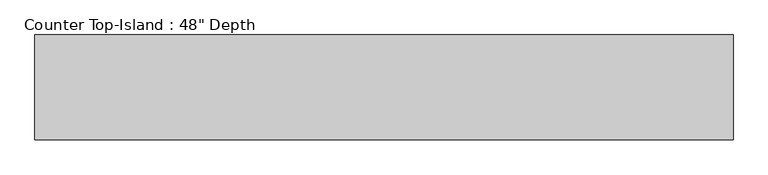
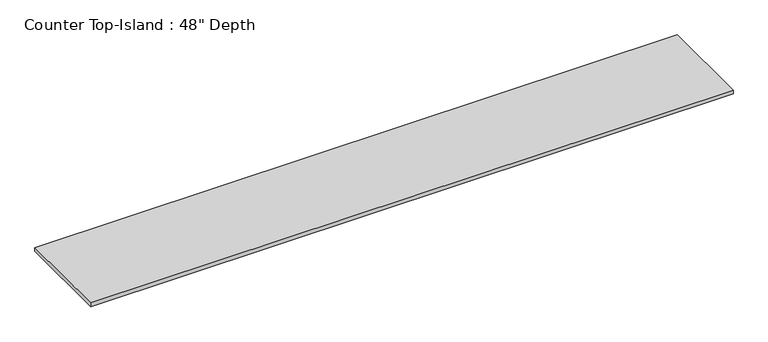
"""IFC4 building model written with IfcOpenShell, lengths in millimetres: furniture geometry."""

from ifc_helpers import new_model, si_unit, frame, origin, place, context, project, spatial, polyline, outline, extrude, source, transform, mapped, element, save


def furniture_cfc005fb(model_context):
    return source(origin(), model_context, "Body", "SweptSolid", [
        extrude(outline(polyline([(4895.5377049, 25.4), (4895.5377049, -889.0), (-1200.4622951, -889.0), (-1200.4622951, 25.4), (4895.5377049, 25.4)])), frame((0.0, 0.0, -38.1), z_axis=(0.0, 0.0, 1.0), x_axis=(1.0, 0.0, 0.0)), (0.0, 0.0, 1.0), 38.1),
    ])


if __name__ == "__main__":
    model = new_model("IFC4")
    model_context = context("Model", 3, world=origin())
    ifc_project = project(units=[si_unit("LENGTHUNIT", "METRE", prefix="MILLI")], contexts=[model_context])
    site = spatial("IfcSite", under=ifc_project)
    building = spatial("IfcBuilding", under=site)
    placement = place(None, origin())
    furniture_shape = furniture_cfc005fb(model_context)
    element("IfcFurniture", 1, ObjectType="Counter Top-Island : 48\" Depth", at=placement, inside=building, context=model_context, shape_type="MappedRepresentation", body=[
        mapped(furniture_shape, transform((0.0, 0.0, 0.0), x_axis=(1.0, 0.0, 0.0), y_axis=(0.0, 1.0, 0.0), z_axis=(0.0, 0.0, 1.0))),
    ])
    save(model, "model.ifc")

# Revit data of these elements
# Type "Counter Top-Island : 48\" Depth"
#   Assembly Code = "C1030400"
#   Width = 3' - 0"
#   Counter Thickness = 0' - 1 1/2"
#   Depth [instance default] = 4' - 2"
#   Length [instance default] = 8' - 0"
#   Counter Top Material = none
#   Default Elevation = 0
#   Height = 0
# Element 1 (IfcFurniture, "Counter Top-Island : 48\" Depth")
#   Depth = 3' - 0"
#   Length = 20' - 0"
#   Materials on its faces: "Counter Top"
# Materials
#   "Counter Top": class "Wood", colour RGB 226 177 128, transparency 0
